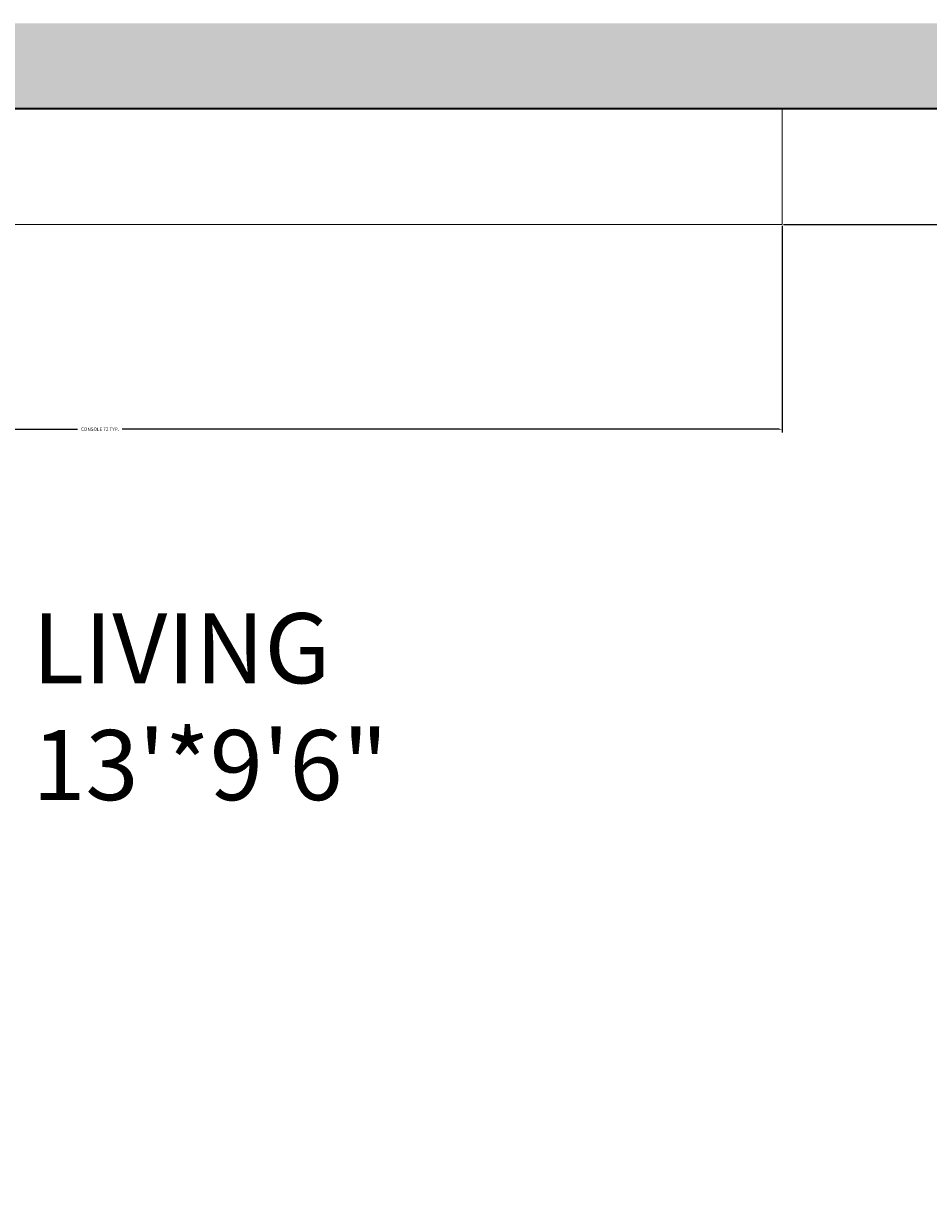
# Model space of a CAD drawing. Units: inches. Extents: x 1998 to 2588, y 1139 to 1977.
# Tile 129 of 134: x 2441 to 2489, y 1698 to 1760. Entities that reach past the tile are written whole.
import ezdxf

# ---------------------------------------------------------------- set-up
doc = ezdxf.new("R2010")
doc.units = ezdxf.units.IN
for name, color, linetype, lineweight in [('A-ANNO-DIMS', 2, 'Continuous', 18), ('A-AREA-IDEN', 7, 'Continuous', 18), ('A-WALL-PATT', 252, 'Continuous', 13), ('FUR', 21, 'Continuous', 18), ('WALL', 200, 'Continuous', 35)]:
    doc.layers.add(name, color=color, linetype=linetype, lineweight=lineweight)
doc.styles.get("Standard").update_dxf_attribs({"font": 'arial.ttf'})
doc.dimstyles.get("Standard").update_dxf_attribs({"dimtxt": 0.18, "dimasz": 0.18, "dimexe": 0.18, "dimexo": 0.0625, "dimgap": 0.09, "dimtad": 0, "dimtih": 1, "dimtoh": 1, "dimdec": 4, "dimzin": 0, "dimdsep": 46, "dimtxsty": 'Standard', "dimcen": 0.09, "dimadec": 0, "dimazin": 0, "dimtfac": 1, "dimtdec": 4, "dimtofl": 0, "dimtmove": 0, "dimatfit": 3, "dimfxl": 1, "dimtolj": 1, "dimtzin": 0, "dimarcsym": 0})

# ---------------------------------------------------------------- blocks, each defined once
blk = doc.blocks.new('CONSOLE-WALL')
blk.add_lwpolyline([(0, 6.123), (71.98, 6.123), (71.98, 0), (0, 0)], close=True)
blk = doc.blocks.new('*D17')
at = {"layer": 'A-ANNO-DIMS', "color": 0, "lineweight": -2, "transparency": 16777216}
for p, q in [((2409.062, 1749.046), (2409.062, 1738.132)), ((2481.042, 1749.046), (2481.042, 1738.132)), ((2409.242, 1738.312), (2443.875, 1738.312)), ((2480.862, 1738.312), (2446.228, 1738.312))]:
    blk.add_line(p, q, dxfattribs=at)
at = {"layer": 'A-ANNO-DIMS', "color": 0, "transparency": 16777216}
for points in [[(2409.242, 1738.342), (2409.242, 1738.282), (2409.062, 1738.312)], [(2480.862, 1738.342), (2480.862, 1738.282), (2481.042, 1738.312)]]:
    blk.add_solid(points, dxfattribs=at)
at = {"layer": 'Defpoints', "color": 0, "transparency": 16777216}
for p in [(2409.062, 1749.109), (2481.042, 1749.109), (2481.042, 1738.312)]:
    blk.add_point(p, dxfattribs=at)
at = {"layer": 'A-ANNO-DIMS', "color": 0, "transparency": 16777216, "insert": (2445.052, 1738.312), "char_height": 0.18, "attachment_point": 5}
blk.add_mtext('\\A1;CONSOLE 72 TYP.', dxfattribs=at)
blk = doc.blocks.new('*D18')
at = {"layer": 'A-ANNO-DIMS', "color": 0, "lineweight": -2, "transparency": 16777216}
for p, q in [((2481.104, 1755.232), (2492.018, 1755.232)), ((2491.838, 1755.052), (2491.838, 1752.353)), ((2491.838, 1749.289), (2491.838, 1751.989)), ((2481.104, 1749.109), (2492.018, 1749.109))]:
    blk.add_line(p, q, dxfattribs=at)
at = {"layer": 'A-ANNO-DIMS', "color": 0, "transparency": 16777216}
for points in [[(2491.808, 1755.052), (2491.868, 1755.052), (2491.838, 1755.232)], [(2491.808, 1749.289), (2491.868, 1749.289), (2491.838, 1749.109)]]:
    blk.add_solid(points, dxfattribs=at)
at = {"layer": 'Defpoints', "color": 0, "transparency": 16777216}
for p in [(2481.042, 1755.232), (2491.838, 1755.232), (2481.042, 1749.109)]:
    blk.add_point(p, dxfattribs=at)
at = {"layer": 'A-ANNO-DIMS', "color": 0, "transparency": 16777216, "insert": (2491.838, 1752.171), "char_height": 0.18, "attachment_point": 5}
blk.add_mtext('\\A1;6 TYP.', dxfattribs=at)
blk = doc.blocks.new('*D24')
at = {"layer": 'A-ANNO-DIMS', "color": 0, "lineweight": -2, "transparency": 16777216}
for p, q in [((2398.535, 1911.232), (2588.309, 1911.232)), ((2588.129, 1911.052), (2588.129, 1570.164)), ((2588.129, 1228.912), (2588.129, 1569.8)), ((2527.535, 1228.732), (2588.309, 1228.732))]:
    blk.add_line(p, q, dxfattribs=at)
at = {"layer": 'A-ANNO-DIMS', "color": 0, "transparency": 16777216}
for points in [[(2588.099, 1911.052), (2588.159, 1911.052), (2588.129, 1911.232)], [(2588.099, 1228.912), (2588.159, 1228.912), (2588.129, 1228.732)]]:
    blk.add_solid(points, dxfattribs=at)
at = {"layer": 'Defpoints', "color": 0, "transparency": 16777216}
for p in [(2398.473, 1911.232), (2588.129, 1911.232), (2527.473, 1228.732)]:
    blk.add_point(p, dxfattribs=at)
at = {"layer": 'A-ANNO-DIMS', "color": 0, "transparency": 16777216, "insert": (2588.129, 1569.982), "char_height": 0.18, "attachment_point": 5}
blk.add_mtext('\\A1;682.5', dxfattribs=at)

msp = doc.modelspace()

# ---------------------------------------------------------------- hatches: boundary and pattern name
at = {"layer": 'A-WALL-PATT'}
h = msp.add_hatch(color=256, dxfattribs=at)
h.dxf.hatch_style = 1
h.paths.add_polyline_path([(2227.4729, 1911.2324), (2222.9729, 1911.2324), (2222.9729, 1888.7324), (2227.4729, 1888.7324)])
h.paths.add_polyline_path([(2236.4493, 1870.3636), (2236.4493, 1875.2324), (2234.4125, 1875.2324), (2234.4125, 1868.3278), (2227.4729, 1868.3278), (2227.4729, 1866.2324), (2236.4493, 1866.2324)])
h.paths.add_polyline_path([(2330.0332, 1875.2324), (2263.9907, 1875.2324), (2263.9907, 1866.2324), (2330.0332, 1866.2324)])
h.paths.add_polyline_path([(2345.9729, 1906.7324), (2393.9729, 1906.7324), (2393.9729, 1882.7324), (2345.9729, 1882.7324), (2345.9729, 1878.2324), (2393.9729, 1878.2324), (2398.4729, 1878.2324), (2398.4729, 1882.7324), (2398.4729, 1911.2324), (2345.9729, 1911.2324), (2341.4729, 1911.2324), (2341.4729, 1866.2324), (2341.4729, 1790.0412), (2345.9729, 1790.0412), (2345.9729, 1875.2324)])
h.paths.add_polyline_path([(2398.4729, 1878.2324), (2393.9729, 1878.2324), (2393.9729, 1798.2324), (2393.9729, 1793.7324), (2398.4729, 1793.7324)], flags=17)
h.paths.add_polyline_path([(2393.9729, 1798.2324), (2375.7311, 1798.2324, -0.005968), (2375.7384, 1797.6146), (2375.7384, 1793.7324), (2393.9729, 1793.7324)], flags=17)
h.paths.add_polyline_path([(2349.8569, 1797.6146), (2349.8569, 1798.2324), (2345.9729, 1798.2324), (2345.9729, 1793.7324), (2349.8569, 1793.7324)], flags=17)
h.paths.add_polyline_path([(2398.4729, 1793.7324), (2393.9729, 1793.7324), (2393.9729, 1790.0412), (2398.4729, 1790.0412)], flags=17)
h.paths.add_polyline_path([(2527.4729, 1882.7324), (2507.8006, 1882.7324), (2507.8006, 1878.2324), (2518.4729, 1878.2324), (2518.4729, 1759.7324), (2510.9729, 1759.7324), (2510.9729, 1755.2324), (2527.4729, 1755.2324)])
h.paths.add_polyline_path([(2487.396, 1882.7324), (2398.4729, 1882.7324), (2398.4729, 1878.2324), (2487.396, 1878.2324)])
h.paths.add_polyline_path([(2490.5682, 1759.7324), (2345.9729, 1759.7324), (2345.9729, 1755.2324), (2490.5682, 1755.2324)])
h.paths.add_polyline_path([(2398.4729, 1760.5844), (2398.3914, 1760.5844), (2393.9729, 1760.5844), (2393.9729, 1759.7324), (2398.4729, 1759.7324)])
h.paths.add_polyline_path([(2334.5332, 1759.7324), (2234.4125, 1759.7324), (2234.4125, 1755.2324), (2334.5332, 1755.2324)])
h.paths.add_polyline_path([(2345.9729, 1760.5844), (2341.5543, 1760.5844), (2341.4729, 1760.5844), (2341.4729, 1759.7324), (2345.9729, 1759.7324)])
h.paths.add_polyline_path([(2222.9729, 1759.7324), (2221.7204, 1759.7324), (2221.7204, 1755.2324), (2222.9729, 1755.2324)])
h.paths.add_polyline_path([(2061.4729, 1702.7324), (2059.4729, 1702.7324), (2059.4729, 1584.2324), (2061.4729, 1584.2324)])
h.paths.add_polyline_path([(2061.4729, 1584.2324), (2059.4729, 1584.2324), (2059.4729, 1470.2324), (2061.4729, 1470.2324)])
h.paths.add_polyline_path([(2510.9729, 1469.2927), (2501.9729, 1469.2927), (2501.9729, 1369.172), (2510.9729, 1369.172)])
h.paths.add_polyline_path([(2227.4729, 1369.7324), (2227.4729, 1417.7324), (2221.4126, 1417.7324), (2221.4126, 1413.2324), (2222.9729, 1413.2324), (2222.9729, 1293.2324), (2222.9729, 1285.137), (2227.4729, 1285.137)])

# ---------------------------------------------------------------- linework, layer by layer
at = {"layer": 'WALL'}
for q in [(2527.4729, 1755.2324), (2501.9729, 1755.2324)]:
    msp.add_line((2345.9729, 1755.2324), q, dxfattribs=at)

# ---------------------------------------------------------------- block references
at = {"layer": 'FUR'}
msp.add_blockref('CONSOLE-WALL', (2409.062, 1749.109), dxfattribs=at)

# ---------------------------------------------------------------- texts
at = {"layer": 'A-AREA-IDEN', "insert": (2441.4826, 1728.6031), "char_height": 3.69875, "attachment_point": 1}
msp.add_mtext_dynamic_manual_height_columns('LIVING\\P13\'*9\'6"', width=110.572713, gutter_width=18.4938, heights=[0], dxfattribs=at)

# ---------------------------------------------------------------- dimensions: what is measured, and where the dimension line sits
at = {"layer": 'A-ANNO-DIMS'}
dim = msp.add_linear_dim(base=(2588.1286, 1911.2324), p1=(2527.4729, 1228.7324), p2=(2398.4729, 1911.2324), angle=90, dimstyle='Standard', override={"dimdec": 1, "dimlfac": 1, "dimrnd": 0, "dimzin": 0, "dimdsep": 46, "dimlunit": 2}, dxfattribs=at)
dim.commit()
dim.dimension.update_dxf_attribs({"geometry": '*D24', "text_midpoint": (2588.1286, 1569.9824)})
dim = msp.add_linear_dim(base=(2491.8385, 1755.2324), p1=(2481.0415, 1749.1089), p2=(2481.0415, 1755.2324), angle=90, text='<> TYP.', dimstyle='Standard', override={"dimdec": 0, "dimlfac": 1, "dimrnd": 0, "dimzin": 0, "dimdsep": 46, "dimlunit": 2}, dxfattribs=at)
dim.commit()
dim.dimension.update_dxf_attribs({"geometry": '*D18', "text_midpoint": (2491.8385, 1752.1707)})
dim = msp.add_linear_dim(base=(2481.0415, 1738.312), p1=(2409.0618, 1749.1089), p2=(2481.0415, 1749.1089), text='CONSOLE <> TYP.', dimstyle='Standard', override={"dimdec": 0, "dimlfac": 1, "dimrnd": 0, "dimzin": 0, "dimdsep": 46, "dimlunit": 2}, dxfattribs=at)
dim.commit()
dim.dimension.update_dxf_attribs({"geometry": '*D17', "text_midpoint": (2445.0517, 1738.312)})

doc.saveas('drawing.dxf')
